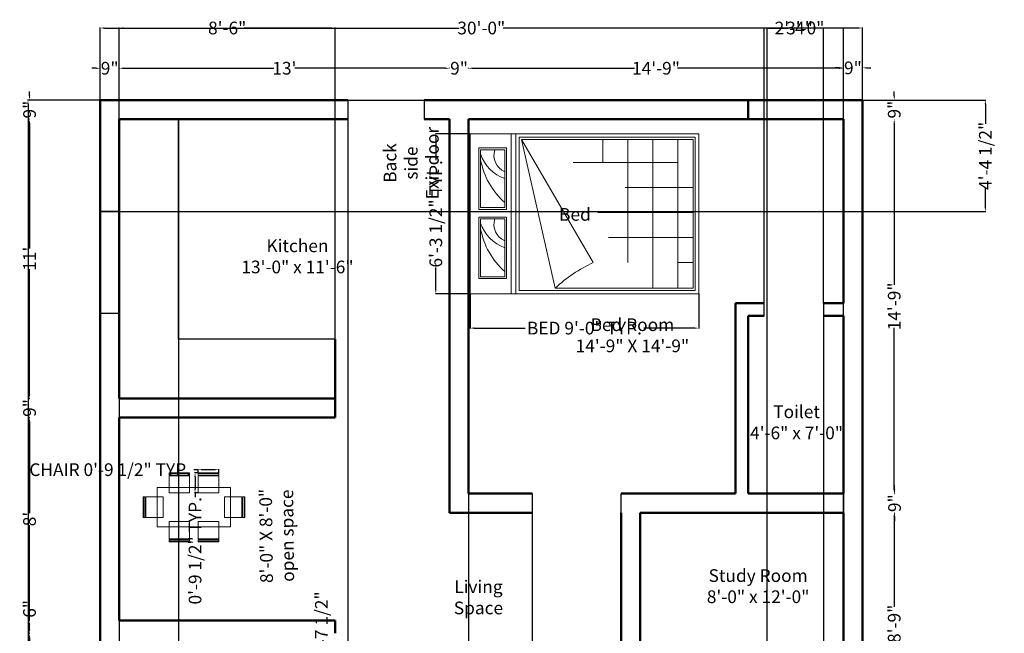
# Model space of a CAD drawing. Units: inches. Extents: x 35 to 505, y 81 to 785.
# Tile 3 of 3: x 40 to 505, y 495 to 785. Entities that reach past the tile are written whole.
import ezdxf

# ---------------------------------------------------------------- set-up
doc = ezdxf.new("R2010")
doc.units = ezdxf.units.IN
doc.header["$MEASUREMENT"] = 0
for name, color, linetype, lineweight in [('A-ANNO-DIMS', 2, 'Continuous', 13), ('A-ANNO-TEXT', 7, 'Continuous', 18), ('A-AREA-IDEN', 7, 'Continuous', 20), ('A-DOOR', 3, 'Continuous', 30), ('A-FLOR-CASE', 8, 'Continuous', 25), ('A-FURN', 6, 'Continuous', 18), ('A-GLAZ', 4, 'Continuous', 25), ('A-WALL', 7, 'Continuous', 50)]:
    doc.layers.add(name, color=color, linetype=linetype, lineweight=lineweight)
doc.styles.get("Standard").update_dxf_attribs({"font": 'arial.ttf'})
doc.dimstyles.get("Standard").update_dxf_attribs({"dimtxt": 6, "dimasz": 2, "dimexe": 0.18, "dimexo": 0.0625, "dimgap": 0.09, "dimtad": 0, "dimdec": 0, "dimzin": 0, "dimdsep": 46, "dimlunit": 4, "dimtxsty": 'Standard', "dimcen": 0.09, "dimadec": 0, "dimazin": 0, "dimtfac": 1, "dimtdec": 0, "dimtofl": 0, "dimtmove": 0, "dimatfit": 3, "dimfxl": 1, "dimtolj": 1, "dimtzin": 0, "dimarcsym": 0})

# ---------------------------------------------------------------- blocks, each defined once
blk = doc.blocks.new('*D6')
at = {"layer": 'A-ANNO-DIMS', "color": 0, "lineweight": -2, "transparency": 16777216}
for p, q in [((44.65, 495.11), (44.53, 495.11)), ((44.71, 493.11), (44.71, 474.08)), ((44.71, 449.11), (44.71, 468.14)), ((44.71, 447.11), (44.89, 447.11))]:
    blk.add_line(p, q, dxfattribs=at)
at = {"layer": 'A-ANNO-DIMS', "color": 0, "transparency": 16777216}
for points in [[(44.38, 493.11), (45.04, 493.11), (44.71, 495.11)], [(44.38, 449.11), (45.04, 449.11), (44.71, 447.11)]]:
    blk.add_solid(points, dxfattribs=at)
at = {"layer": 'Defpoints', "color": 0, "transparency": 16777216}
for p in [(44.71, 495.11), (44.71, 495.11), (44.65, 447.11)]:
    blk.add_point(p, dxfattribs=at)
at = {"layer": 'A-ANNO-DIMS', "color": 0, "transparency": 16777216, "insert": (44.71, 471.11), "char_height": 6, "attachment_point": 5, "rotation": 90}
blk.add_mtext("\\A1;4'", dxfattribs=at)
blk = doc.blocks.new('*D7')
at = {"layer": 'A-ANNO-DIMS', "color": 0, "lineweight": -2, "transparency": 16777216}
for p, q in [((44.71, 501.11), (44.71, 503.11)), ((44.65, 501.11), (44.53, 501.11)), ((44.71, 497.11), (44.71, 499.11)), ((44.77, 495.11), (44.89, 495.11))]:
    blk.add_line(p, q, dxfattribs=at)
at = {"layer": 'A-ANNO-DIMS', "color": 0, "transparency": 16777216}
for points in [[(44.38, 499.11), (45.04, 499.11), (44.71, 501.11)], [(44.38, 497.11), (45.04, 497.11), (44.71, 495.11)]]:
    blk.add_solid(points, dxfattribs=at)
at = {"layer": 'Defpoints', "color": 0, "transparency": 16777216}
for p in [(44.71, 501.11), (44.71, 501.11), (44.71, 495.11)]:
    blk.add_point(p, dxfattribs=at)
at = {"layer": 'A-ANNO-DIMS', "color": 0, "transparency": 16777216, "insert": (44.71, 506.66), "char_height": 6, "attachment_point": 5, "rotation": 90}
blk.add_mtext('\\A1;6"', dxfattribs=at)
blk = doc.blocks.new('*D8')
at = {"layer": 'A-ANNO-DIMS', "color": 0, "lineweight": -2, "transparency": 16777216}
for p, q in [((44.65, 597.11), (44.53, 597.11)), ((44.71, 595.11), (44.71, 551.96)), ((44.71, 503.11), (44.71, 546.25)), ((44.77, 501.11), (44.89, 501.11))]:
    blk.add_line(p, q, dxfattribs=at)
at = {"layer": 'A-ANNO-DIMS', "color": 0, "transparency": 16777216}
for points in [[(44.38, 595.11), (45.04, 595.11), (44.71, 597.11)], [(44.38, 503.11), (45.04, 503.11), (44.71, 501.11)]]:
    blk.add_solid(points, dxfattribs=at)
at = {"layer": 'Defpoints', "color": 0, "transparency": 16777216}
for p in [(44.71, 597.11), (44.71, 597.11), (44.71, 501.11)]:
    blk.add_point(p, dxfattribs=at)
at = {"layer": 'A-ANNO-DIMS', "color": 0, "transparency": 16777216, "insert": (44.71, 549.11), "char_height": 6, "attachment_point": 5, "rotation": 90}
blk.add_mtext("\\A1;8'", dxfattribs=at)
blk = doc.blocks.new('*D9')
at = {"layer": 'A-ANNO-DIMS', "color": 0, "lineweight": -2, "transparency": 16777216}
for p, q in [((44.71, 608.11), (44.71, 610.11)), ((44.65, 606.11), (44.53, 606.11)), ((44.59, 597.11), (44.89, 597.11)), ((44.71, 595.11), (44.71, 593.11))]:
    blk.add_line(p, q, dxfattribs=at)
at = {"layer": 'A-ANNO-DIMS', "color": 0, "transparency": 16777216}
for points in [[(44.38, 608.11), (45.04, 608.11), (44.71, 606.11)], [(44.38, 595.11), (45.04, 595.11), (44.71, 597.11)]]:
    blk.add_solid(points, dxfattribs=at)
at = {"layer": 'Defpoints', "color": 0, "transparency": 16777216}
for p in [(44.71, 606.11), (44.53, 597.11), (44.71, 597.11)]:
    blk.add_point(p, dxfattribs=at)
at = {"layer": 'A-ANNO-DIMS', "color": 0, "transparency": 16777216, "insert": (44.71, 601.61), "char_height": 6, "attachment_point": 5, "rotation": 90}
blk.add_mtext('\\A1;9"', dxfattribs=at)
blk = doc.blocks.new('*D10')
at = {"layer": 'A-ANNO-DIMS', "color": 0, "lineweight": -2, "transparency": 16777216}
for p, q in [((44.65, 738.11), (44.53, 738.11)), ((44.71, 736.11), (44.71, 677.01)), ((44.71, 608.11), (44.71, 667.21)), ((44.77, 606.11), (44.89, 606.11))]:
    blk.add_line(p, q, dxfattribs=at)
at = {"layer": 'A-ANNO-DIMS', "color": 0, "transparency": 16777216}
for points in [[(44.38, 736.11), (45.04, 736.11), (44.71, 738.11)], [(44.38, 608.11), (45.04, 608.11), (44.71, 606.11)]]:
    blk.add_solid(points, dxfattribs=at)
at = {"layer": 'Defpoints', "color": 0, "transparency": 16777216}
for p in [(44.71, 738.11), (44.71, 738.11), (44.71, 606.11)]:
    blk.add_point(p, dxfattribs=at)
at = {"layer": 'A-ANNO-DIMS', "color": 0, "transparency": 16777216, "insert": (44.71, 672.11), "char_height": 6, "attachment_point": 5, "rotation": 90}
blk.add_mtext("\\A1;11'", dxfattribs=at)
blk = doc.blocks.new('*D11')
at = {"layer": 'A-ANNO-DIMS', "color": 0, "lineweight": -2, "transparency": 16777216}
for p, q in [((44.71, 749.11), (44.71, 751.11)), ((44.65, 747.11), (44.53, 747.11)), ((44.65, 738.11), (44.53, 738.11)), ((44.71, 736.11), (44.71, 734.11))]:
    blk.add_line(p, q, dxfattribs=at)
at = {"layer": 'A-ANNO-DIMS', "color": 0, "transparency": 16777216}
for points in [[(44.38, 749.11), (45.04, 749.11), (44.71, 747.11)], [(44.38, 736.11), (45.04, 736.11), (44.71, 738.11)]]:
    blk.add_solid(points, dxfattribs=at)
at = {"layer": 'Defpoints', "color": 0, "transparency": 16777216}
for p in [(44.71, 747.11), (44.71, 738.11), (44.71, 738.11)]:
    blk.add_point(p, dxfattribs=at)
at = {"layer": 'A-ANNO-DIMS', "color": 0, "transparency": 16777216, "insert": (44.71, 742.61), "char_height": 6, "attachment_point": 5, "rotation": 90}
blk.add_mtext('\\A1;9"', dxfattribs=at)
blk = doc.blocks.new('*D12')
at = {"layer": 'A-ANNO-DIMS', "color": 0, "lineweight": -2, "transparency": 16777216}
for p, q in [((76.06, 762.14), (74.06, 762.14)), ((78.06, 747.17), (78.06, 762.32)), ((87.06, 762.21), (87.06, 762.32)), ((89.06, 762.14), (91.06, 762.14))]:
    blk.add_line(p, q, dxfattribs=at)
at = {"layer": 'A-ANNO-DIMS', "color": 0, "transparency": 16777216}
for points in [[(76.06, 762.48), (76.06, 761.81), (78.06, 762.14)], [(89.06, 762.48), (89.06, 761.81), (87.06, 762.14)]]:
    blk.add_solid(points, dxfattribs=at)
at = {"layer": 'Defpoints', "color": 0, "transparency": 16777216}
for p in [(78.06, 762.14), (87.06, 762.14), (78.06, 747.11)]:
    blk.add_point(p, dxfattribs=at)
at = {"layer": 'A-ANNO-DIMS', "color": 0, "transparency": 16777216, "insert": (82.56, 762.14), "char_height": 6, "attachment_point": 5}
blk.add_mtext('\\A1;9"', dxfattribs=at)
blk = doc.blocks.new('*D13')
at = {"layer": 'A-ANNO-DIMS', "color": 0, "lineweight": -2, "transparency": 16777216}
for p, q in [((87.06, 762.26), (87.06, 761.96)), ((89.06, 762.14), (160.16, 762.14)), ((241.06, 762.14), (169.96, 762.14)), ((243.06, 762.21), (243.06, 762.32))]:
    blk.add_line(p, q, dxfattribs=at)
at = {"layer": 'A-ANNO-DIMS', "color": 0, "transparency": 16777216}
for points in [[(89.06, 762.48), (89.06, 761.81), (87.06, 762.14)], [(241.06, 762.48), (241.06, 761.81), (243.06, 762.14)]]:
    blk.add_solid(points, dxfattribs=at)
at = {"layer": 'Defpoints', "color": 0, "transparency": 16777216}
for p in [(87.06, 762.32), (243.06, 762.14), (243.06, 762.14)]:
    blk.add_point(p, dxfattribs=at)
at = {"layer": 'A-ANNO-DIMS', "color": 0, "transparency": 16777216, "insert": (165.06, 762.14), "char_height": 6, "attachment_point": 5}
blk.add_mtext("\\A1;13'", dxfattribs=at)
blk = doc.blocks.new('*D14')
at = {"layer": 'A-ANNO-DIMS', "color": 0, "lineweight": -2, "transparency": 16777216}
for p, q in [((241.06, 762.14), (239.06, 762.14)), ((243.06, 762.21), (243.06, 762.32)), ((252.06, 762.21), (252.06, 762.32)), ((254.06, 762.14), (256.06, 762.14))]:
    blk.add_line(p, q, dxfattribs=at)
at = {"layer": 'A-ANNO-DIMS', "color": 0, "transparency": 16777216}
for points in [[(241.06, 762.48), (241.06, 761.81), (243.06, 762.14)], [(254.06, 762.48), (254.06, 761.81), (252.06, 762.14)]]:
    blk.add_solid(points, dxfattribs=at)
at = {"layer": 'Defpoints', "color": 0, "transparency": 16777216}
for p in [(243.06, 762.14), (252.06, 762.14), (252.06, 762.14)]:
    blk.add_point(p, dxfattribs=at)
at = {"layer": 'A-ANNO-DIMS', "color": 0, "transparency": 16777216, "insert": (247.56, 762.14), "char_height": 6, "attachment_point": 5}
blk.add_mtext('\\A1;9"', dxfattribs=at)
blk = doc.blocks.new('*D15')
at = {"layer": 'A-ANNO-DIMS', "color": 0, "lineweight": -2, "transparency": 16777216}
for p, q in [((252.06, 762.26), (252.06, 761.96)), ((254.06, 762.14), (330.44, 762.14)), ((427.06, 762.14), (350.67, 762.14)), ((429.06, 762.21), (429.06, 762.32))]:
    blk.add_line(p, q, dxfattribs=at)
at = {"layer": 'A-ANNO-DIMS', "color": 0, "transparency": 16777216}
for points in [[(254.06, 762.48), (254.06, 761.81), (252.06, 762.14)], [(427.06, 762.48), (427.06, 761.81), (429.06, 762.14)]]:
    blk.add_solid(points, dxfattribs=at)
at = {"layer": 'Defpoints', "color": 0, "transparency": 16777216}
for p in [(252.06, 762.32), (429.06, 762.14), (429.06, 762.14)]:
    blk.add_point(p, dxfattribs=at)
at = {"layer": 'A-ANNO-DIMS', "color": 0, "transparency": 16777216, "insert": (340.56, 762.14), "char_height": 6, "attachment_point": 5}
blk.add_mtext('\\A1;14\'-9"', dxfattribs=at)
blk = doc.blocks.new('*D16')
at = {"layer": 'A-ANNO-DIMS', "color": 0, "lineweight": -2, "transparency": 16777216}
for p, q in [((427.06, 762.32), (425.06, 762.32)), ((429.06, 762.21), (429.06, 762.5)), ((438.06, 747.17), (438.06, 762.5)), ((440.06, 762.32), (442.06, 762.32))]:
    blk.add_line(p, q, dxfattribs=at)
at = {"layer": 'A-ANNO-DIMS', "color": 0, "transparency": 16777216}
for points in [[(427.06, 762.66), (427.06, 761.99), (429.06, 762.32)], [(440.06, 762.66), (440.06, 761.99), (438.06, 762.32)]]:
    blk.add_solid(points, dxfattribs=at)
at = {"layer": 'Defpoints', "color": 0, "transparency": 16777216}
for p in [(429.06, 762.14), (438.06, 762.32), (438.06, 747.11)]:
    blk.add_point(p, dxfattribs=at)
at = {"layer": 'A-ANNO-DIMS', "color": 0, "transparency": 16777216, "insert": (433.56, 762.32), "char_height": 6, "attachment_point": 5}
blk.add_mtext('\\A1;9"', dxfattribs=at)
blk = doc.blocks.new('*D22')
at = {"layer": 'A-ANNO-DIMS', "color": 0, "lineweight": -2, "transparency": 16777216}
for p, q in [((453.06, 749.11), (453.06, 751.11)), ((438.12, 747.11), (453.24, 747.11)), ((453.06, 736.11), (453.06, 734.11)), ((453.12, 738.11), (453.24, 738.11))]:
    blk.add_line(p, q, dxfattribs=at)
at = {"layer": 'A-ANNO-DIMS', "color": 0, "transparency": 16777216}
for points in [[(452.72, 749.11), (453.39, 749.11), (453.06, 747.11)], [(452.72, 736.11), (453.39, 736.11), (453.06, 738.11)]]:
    blk.add_solid(points, dxfattribs=at)
at = {"layer": 'Defpoints', "color": 0, "transparency": 16777216}
for p in [(438.06, 747.11), (453.06, 738.11), (453.06, 738.11)]:
    blk.add_point(p, dxfattribs=at)
at = {"layer": 'A-ANNO-DIMS', "color": 0, "transparency": 16777216, "insert": (453.06, 742.61), "char_height": 6, "attachment_point": 5, "rotation": 90}
blk.add_mtext('\\A1;9"', dxfattribs=at)
blk = doc.blocks.new('*D23')
at = {"layer": 'A-ANNO-DIMS', "color": 0, "lineweight": -2, "transparency": 16777216}
for p, q in [((453.06, 736.11), (453.06, 659.72)), ((453.12, 738.11), (453.24, 738.11)), ((453.06, 563.11), (453.06, 639.5)), ((453.12, 561.11), (453.24, 561.11))]:
    blk.add_line(p, q, dxfattribs=at)
at = {"layer": 'A-ANNO-DIMS', "color": 0, "transparency": 16777216}
for points in [[(452.72, 736.11), (453.39, 736.11), (453.06, 738.11)], [(452.72, 563.11), (453.39, 563.11), (453.06, 561.11)]]:
    blk.add_solid(points, dxfattribs=at)
at = {"layer": 'Defpoints', "color": 0, "transparency": 16777216}
for p in [(453.06, 738.11), (453.06, 561.11), (453.06, 561.11)]:
    blk.add_point(p, dxfattribs=at)
at = {"layer": 'A-ANNO-DIMS', "color": 0, "transparency": 16777216, "insert": (453.06, 649.61), "char_height": 6, "attachment_point": 5, "rotation": 90}
blk.add_mtext('\\A1;14\'-9"', dxfattribs=at)
blk = doc.blocks.new('*D24')
at = {"layer": 'A-ANNO-DIMS', "color": 0, "lineweight": -2, "transparency": 16777216}
for p, q in [((453.23, 563.11), (453.23, 565.11)), ((453.12, 561.11), (453.41, 561.11)), ((453.12, 552.11), (453.41, 552.11)), ((453.23, 550.11), (453.23, 548.11))]:
    blk.add_line(p, q, dxfattribs=at)
at = {"layer": 'A-ANNO-DIMS', "color": 0, "transparency": 16777216}
for points in [[(452.9, 563.11), (453.56, 563.11), (453.23, 561.11)], [(452.9, 550.11), (453.56, 550.11), (453.23, 552.11)]]:
    blk.add_solid(points, dxfattribs=at)
at = {"layer": 'Defpoints', "color": 0, "transparency": 16777216}
for p in [(453.06, 561.11), (453.06, 552.11), (453.23, 552.11)]:
    blk.add_point(p, dxfattribs=at)
at = {"layer": 'A-ANNO-DIMS', "color": 0, "transparency": 16777216, "insert": (453.23, 556.61), "char_height": 6, "attachment_point": 5, "rotation": 90}
blk.add_mtext('\\A1;9"', dxfattribs=at)
blk = doc.blocks.new('*D25')
at = {"layer": 'A-ANNO-DIMS', "color": 0, "lineweight": -2, "transparency": 16777216}
for p, q in [((453.06, 550.11), (453.06, 507.68)), ((453.12, 552.11), (453.24, 552.11)), ((453.06, 449.11), (453.06, 491.54)), ((453.12, 447.11), (453.24, 447.11))]:
    blk.add_line(p, q, dxfattribs=at)
at = {"layer": 'A-ANNO-DIMS', "color": 0, "transparency": 16777216}
for points in [[(452.72, 550.11), (453.39, 550.11), (453.06, 552.11)], [(452.72, 449.11), (453.39, 449.11), (453.06, 447.11)]]:
    blk.add_solid(points, dxfattribs=at)
at = {"layer": 'Defpoints', "color": 0, "transparency": 16777216}
for p in [(453.06, 552.11), (453.06, 447.11), (453.06, 447.11)]:
    blk.add_point(p, dxfattribs=at)
at = {"layer": 'A-ANNO-DIMS', "color": 0, "transparency": 16777216, "insert": (453.06, 499.61), "char_height": 6, "attachment_point": 5, "rotation": 90}
blk.add_mtext('\\A1;8\'-9"', dxfattribs=at)
blk = doc.blocks.new('bed')
for p, q in [((309.37, 914.01), (309.37, 1021.97)), ((309.37, 1021.97), (384.97, 1021.97)), ((384.97, 1021.97), (384.97, 913.97)), ((316.65, 1017.78), (345.65, 1017.78)), ((316.65, 1004.77), (316.65, 1017.78)), ((317.46, 1016.97), (344.84, 1016.97)), ((317.46, 1005.58), (317.46, 1016.97)), ((344.84, 1016.97), (344.84, 1005.58)), ((345.65, 1017.78), (345.65, 1004.77)), ((349.3, 1017.78), (378.3, 1017.78)), ((349.3, 1004.77), (349.3, 1017.78)), ((350.11, 1016.97), (377.49, 1016.97)), ((350.11, 1005.58), (350.11, 1016.97)), ((377.49, 1016.97), (377.49, 1005.58)), ((378.3, 1017.78), (378.3, 1004.77)), ((345.65, 1004.77), (316.65, 1004.77)), ((344.84, 1005.58), (317.46, 1005.58)), ((378.3, 1004.77), (349.3, 1004.77)), ((377.49, 1005.58), (350.11, 1005.58)), ((309.37, 1002.53), (384.97, 1002.53)), ((309.37, 1000.37), (384.97, 1000.37)), ((310.99, 998.75), (383.35, 998.75)), ((310.99, 915.59), (310.99, 998.75)), ((382.27, 997.67), (312.07, 981.73)), ((382.27, 997.67), (324.17, 963.79)), ((382.27, 997.67), (382.27, 916.67)), ((383.35, 998.75), (383.35, 915.59)), ((312.07, 916.67), (312.07, 981.73)), ((371.46, 923.83), (371.46, 973.35)), ((347.84, 916.67), (347.84, 961.71)), ((371.46, 959.27), (382.27, 959.27)), ((336.02, 916.67), (336.02, 956.58)), ((359.65, 916.67), (359.65, 948.66)), ((324.21, 947.45), (382.27, 947.45)), ((312.07, 935.64), (382.27, 935.64)), ((312.07, 923.83), (382.27, 923.83)), ((324.21, 916.67), (324.21, 923.83)), ((382.27, 916.67), (312.07, 916.67)), ((384.97, 913.97), (309.37, 914.01)), ((383.35, 915.59), (310.99, 915.59))]:
    blk.add_line(p, q)
for centre, radius, start, end in [((346.35, 982.33), 35.21, 100.2734, 138.6774), ((348.52, 999.48), 18.4, 108.0489, 160.6348), ((378.99, 982.33), 35.21, 100.2734, 138.6774), ((381.16, 999.48), 18.4, 108.0489, 160.6348), ((342.22, 1002.22), 8.48, 71.9504, 156.6806), ((374.86, 1002.22), 8.48, 71.9504, 156.6806), ((263.08, 935.62), 67.27, 24.7582, 43.2711)]:
    blk.add_arc(centre, radius, start, end)
blk = doc.blocks.new('CHAIR-DINING')
for p, q in [((0, 9.51, -23.82), (9.73, 9.51, -23.82)), ((0, 1.4, -23.82), (0, 9.51, -23.82)), ((9.73, 9.51, -23.82), (9.73, 1.4, -23.82)), ((9.73, 1.4, -23.82), (0, 1.4, -23.82)), ((9.73, 1.08, -23.82), (0, 1.08, -23.82)), ((0, 1.08, -23.82), (0, 0, -23.82)), ((9.73, 0.33, -23.82), (0, 0.33, -23.82)), ((0, 0, -23.82), (9.73, 0, -23.82)), ((9.73, 0, -23.82), (9.73, 1.08, -23.82))]:
    blk.add_line(p, q)
blk = doc.blocks.new('WIN-48-JAMBS')
for p, q in [((9, 48), (0, 48)), ((0, 0), (9, 0))]:
    blk.add_line(p, q)
blk = doc.blocks.new('DOOR-36-JAMBS')
for p, q in [((0, 9), (0, 0)), ((36, 9), (36, 0))]:
    blk.add_line(p, q)
blk = doc.blocks.new('*D42')
at = {"layer": 'A-ANNO-DIMS', "color": 0, "lineweight": -2, "transparency": 16777216}
for p, q in [((124.34, 572.44), (122.34, 572.44)), ((124.34, 571.04), (124.34, 572.62)), ((132.06, 572.44), (126.34, 572.44)), ((134.06, 571.04), (134.06, 572.62))]:
    blk.add_line(p, q, dxfattribs=at)
at = {"layer": 'A-ANNO-DIMS', "color": 0, "transparency": 16777216}
for points in [[(126.34, 572.77), (126.34, 572.11), (124.34, 572.44)], [(132.06, 572.77), (132.06, 572.11), (134.06, 572.44)]]:
    blk.add_solid(points, dxfattribs=at)
at = {"layer": 'Defpoints', "color": 0, "transparency": 16777216}
for p in [(124.34, 572.44), (124.34, 570.98), (134.06, 570.98)]:
    blk.add_point(p, dxfattribs=at)
at = {"layer": 'A-ANNO-DIMS', "color": 0, "transparency": 16777216, "insert": (82.8, 572.44), "char_height": 6, "attachment_point": 5}
blk.add_mtext('\\A1;CHAIR 0\'-9 1/2" TYP.', dxfattribs=at)
blk = doc.blocks.new('*D43')
at = {"layer": 'A-ANNO-DIMS', "color": 0, "lineweight": -2, "transparency": 16777216}
for p, q in [((124.27, 570.98), (122.7, 570.98)), ((122.88, 568.98), (122.88, 563.48)), ((124.27, 561.48), (122.7, 561.48)), ((122.88, 561.48), (122.88, 559.48))]:
    blk.add_line(p, q, dxfattribs=at)
at = {"layer": 'A-ANNO-DIMS', "color": 0, "transparency": 16777216}
for points in [[(122.54, 568.98), (123.21, 568.98), (122.88, 570.98)], [(122.54, 563.48), (123.21, 563.48), (122.88, 561.48)]]:
    blk.add_solid(points, dxfattribs=at)
at = {"layer": 'Defpoints', "color": 0, "transparency": 16777216}
for p in [(124.34, 570.98), (122.88, 561.48), (124.34, 561.48)]:
    blk.add_point(p, dxfattribs=at)
at = {"layer": 'A-ANNO-DIMS', "color": 0, "transparency": 16777216, "insert": (122.88, 534.11), "char_height": 6, "attachment_point": 5, "rotation": 90}
blk.add_mtext('\\A1;0\'-9 1/2" TYP.', dxfattribs=at)
blk = doc.blocks.new('*D48')
at = {"layer": 'A-ANNO-DIMS', "color": 0, "lineweight": -2, "transparency": 16777216}
for p, q in [((252.77, 655.48), (252.77, 639.16)), ((360.76, 655.48), (360.76, 639.16)), ((254.77, 639.34), (278.74, 639.34)), ((358.76, 639.34), (334.79, 639.34))]:
    blk.add_line(p, q, dxfattribs=at)
at = {"layer": 'A-ANNO-DIMS', "color": 0, "transparency": 16777216}
for points in [[(254.77, 639.67), (254.77, 639.01), (252.77, 639.34)], [(358.76, 639.67), (358.76, 639.01), (360.76, 639.34)]]:
    blk.add_solid(points, dxfattribs=at)
at = {"layer": 'Defpoints', "color": 0, "transparency": 16777216}
for p in [(252.77, 655.54), (360.76, 655.54), (252.77, 639.34)]:
    blk.add_point(p, dxfattribs=at)
at = {"layer": 'A-ANNO-DIMS', "color": 0, "transparency": 16777216, "insert": (306.77, 639.34), "char_height": 6, "attachment_point": 5}
blk.add_mtext('\\A1;BED 9\'-0" TYP.', dxfattribs=at)
blk = doc.blocks.new('*D49')
at = {"layer": 'A-ANNO-DIMS', "color": 0, "lineweight": -2, "transparency": 16777216}
for p, q in [((252.71, 731.14), (236.39, 731.14)), ((236.57, 729.14), (236.57, 718.72)), ((236.57, 657.54), (236.57, 667.95)), ((252.71, 655.54), (236.39, 655.54))]:
    blk.add_line(p, q, dxfattribs=at)
at = {"layer": 'A-ANNO-DIMS', "color": 0, "transparency": 16777216}
for points in [[(236.24, 729.14), (236.9, 729.14), (236.57, 731.14)], [(236.24, 657.54), (236.9, 657.54), (236.57, 655.54)]]:
    blk.add_solid(points, dxfattribs=at)
at = {"layer": 'Defpoints', "color": 0, "transparency": 16777216}
for p in [(236.57, 731.14), (252.77, 731.14), (252.77, 655.54)]:
    blk.add_point(p, dxfattribs=at)
at = {"layer": 'A-ANNO-DIMS', "color": 0, "transparency": 16777216, "insert": (236.57, 693.34), "char_height": 6, "attachment_point": 5, "rotation": 90}
blk.add_mtext('\\A1;6\'-3 1/2" TYP.', dxfattribs=at)
blk = doc.blocks.new('*D50')
at = {"layer": 'A-ANNO-DIMS', "color": 0, "lineweight": -2, "transparency": 16777216}
for p, q in [((182.56, 413.09), (182.56, 415.09)), ((168.89, 413.09), (182.74, 413.09)), ((182.56, 323.55), (182.56, 411.09)), ((168.89, 321.55), (182.74, 321.55))]:
    blk.add_line(p, q, dxfattribs=at)
at = {"layer": 'A-ANNO-DIMS', "color": 0, "transparency": 16777216}
for points in [[(182.23, 411.09), (182.89, 411.09), (182.56, 413.09)], [(182.23, 323.55), (182.89, 323.55), (182.56, 321.55)]]:
    blk.add_solid(points, dxfattribs=at)
at = {"layer": 'Defpoints', "color": 0, "transparency": 16777216}
for p in [(168.83, 413.09), (182.56, 413.09), (168.83, 321.55)]:
    blk.add_point(p, dxfattribs=at)
at = {"layer": 'A-ANNO-DIMS', "color": 0, "transparency": 16777216, "insert": (182.56, 466.23), "char_height": 6, "attachment_point": 5, "rotation": 90}
blk.add_mtext('\\A1;SEATING GROUP 7\'-7 1/2"', dxfattribs=at)
blk = doc.blocks.new('*D52')
at = {"layer": 'A-ANNO-DIMS', "color": 0, "lineweight": -2, "transparency": 16777216}
for p, q in [((78.06, 747.17), (78.06, 781.34)), ((438.06, 747.17), (438.06, 781.34)), ((80.06, 781.16), (247.66, 781.16)), ((436.06, 781.16), (268.45, 781.16))]:
    blk.add_line(p, q, dxfattribs=at)
at = {"layer": 'A-ANNO-DIMS', "color": 0, "transparency": 16777216}
for points in [[(80.06, 781.49), (80.06, 780.83), (78.06, 781.16)], [(436.06, 781.49), (436.06, 780.83), (438.06, 781.16)]]:
    blk.add_solid(points, dxfattribs=at)
at = {"layer": 'Defpoints', "color": 0, "transparency": 16777216}
for p in [(438.06, 781.16), (78.06, 747.11), (438.06, 747.11)]:
    blk.add_point(p, dxfattribs=at)
at = {"layer": 'A-ANNO-DIMS', "color": 0, "transparency": 16777216, "insert": (258.06, 781.16), "char_height": 6, "attachment_point": 5}
blk.add_mtext('\\A1;30\'-0"', dxfattribs=at)
blk = doc.blocks.new('*D53')
at = {"layer": 'A-ANNO-DIMS', "color": 0, "lineweight": -2, "transparency": 16777216}
for p, q in [((77.99, 747.11), (43.83, 747.11)), ((44.01, 745.11), (44.01, 457.5)), ((44.01, 149.11), (44.01, 436.71)), ((77.99, 147.11), (43.83, 147.11))]:
    blk.add_line(p, q, dxfattribs=at)
at = {"layer": 'A-ANNO-DIMS', "color": 0, "transparency": 16777216}
for points in [[(43.67, 745.11), (44.34, 745.11), (44.01, 747.11)], [(43.67, 149.11), (44.34, 149.11), (44.01, 147.11)]]:
    blk.add_solid(points, dxfattribs=at)
at = {"layer": 'Defpoints', "color": 0, "transparency": 16777216}
for p in [(44.01, 747.11), (78.06, 747.11), (78.06, 147.11)]:
    blk.add_point(p, dxfattribs=at)
at = {"layer": 'A-ANNO-DIMS', "color": 0, "transparency": 16777216, "insert": (44.01, 447.11), "char_height": 6, "attachment_point": 5, "rotation": 90}
blk.add_mtext('\\A1;50\'-0"', dxfattribs=at)
blk = doc.blocks.new('*D54')
at = {"layer": 'A-ANNO-DIMS', "color": 0, "lineweight": -2, "transparency": 16777216}
for p, q in [((87.06, 738.05), (87.06, 90.02)), ((195.06, 738.05), (195.06, 90.02)), ((89.06, 90.2), (132.99, 90.2)), ((193.06, 90.2), (149.12, 90.2))]:
    blk.add_line(p, q, dxfattribs=at)
at = {"layer": 'A-ANNO-DIMS', "color": 0, "transparency": 16777216}
for points in [[(89.06, 90.53), (89.06, 89.86), (87.06, 90.2)], [(193.06, 90.53), (193.06, 89.86), (195.06, 90.2)]]:
    blk.add_solid(points, dxfattribs=at)
at = {"layer": 'Defpoints', "color": 0, "transparency": 16777216}
for p in [(87.06, 738.11), (195.06, 738.11), (195.06, 90.2)]:
    blk.add_point(p, dxfattribs=at)
at = {"layer": 'A-ANNO-DIMS', "color": 0, "transparency": 16777216, "insert": (141.06, 90.2), "char_height": 6, "attachment_point": 5}
blk.add_mtext('\\A1;9\'-0"', dxfattribs=at)
blk = doc.blocks.new('*D55')
at = {"layer": 'A-ANNO-DIMS', "color": 0, "lineweight": -2, "transparency": 16777216}
for p, q in [((78.12, 747.11), (496.29, 747.11)), ((496.11, 745.11), (496.11, 735.93)), ((496.11, 696.4), (496.11, 705.58)), ((78.12, 694.4), (496.29, 694.4))]:
    blk.add_line(p, q, dxfattribs=at)
at = {"layer": 'A-ANNO-DIMS', "color": 0, "transparency": 16777216}
for points in [[(495.77, 745.11), (496.44, 745.11), (496.11, 747.11)], [(495.77, 696.4), (496.44, 696.4), (496.11, 694.4)]]:
    blk.add_solid(points, dxfattribs=at)
at = {"layer": 'Defpoints', "color": 0, "transparency": 16777216}
for p in [(78.06, 747.11), (78.06, 694.4), (496.11, 694.4)]:
    blk.add_point(p, dxfattribs=at)
at = {"layer": 'A-ANNO-DIMS', "color": 0, "transparency": 16777216, "insert": (496.11, 720.75), "char_height": 6, "attachment_point": 5, "rotation": 90}
blk.add_mtext('\\A1;4\'-4 1/2"', dxfattribs=at)
blk = doc.blocks.new('*D60')
at = {"layer": 'A-ANNO-DIMS', "color": 0, "lineweight": -2, "transparency": 16777216}
for p, q in [((87.06, 606.17), (87.06, 781.34)), ((189.06, 606.17), (189.06, 781.34)), ((89.06, 781.16), (129.99, 781.16)), ((187.06, 781.16), (146.13, 781.16))]:
    blk.add_line(p, q, dxfattribs=at)
at = {"layer": 'A-ANNO-DIMS', "color": 0, "transparency": 16777216}
for points in [[(89.06, 781.49), (89.06, 780.83), (87.06, 781.16)], [(187.06, 781.49), (187.06, 780.83), (189.06, 781.16)]]:
    blk.add_solid(points, dxfattribs=at)
at = {"layer": 'Defpoints', "color": 0, "transparency": 16777216}
for p in [(189.06, 781.16), (87.06, 606.11), (189.06, 606.11)]:
    blk.add_point(p, dxfattribs=at)
at = {"layer": 'A-ANNO-DIMS', "color": 0, "transparency": 16777216, "insert": (138.06, 781.16), "char_height": 6, "attachment_point": 5}
blk.add_mtext('\\A1;8\'-6"', dxfattribs=at)
blk = doc.blocks.new('*D61')
at = {"layer": 'A-ANNO-DIMS', "color": 0, "lineweight": -2, "transparency": 16777216}
for p, q in [((87.06, 738.05), (87.06, 90.02)), ((115.06, 738.05), (115.06, 90.02)), ((89.06, 90.2), (92.94, 90.2)), ((113.06, 90.2), (109.17, 90.2))]:
    blk.add_line(p, q, dxfattribs=at)
at = {"layer": 'A-ANNO-DIMS', "color": 0, "transparency": 16777216}
for points in [[(89.06, 90.53), (89.06, 89.86), (87.06, 90.2)], [(113.06, 90.53), (113.06, 89.86), (115.06, 90.2)]]:
    blk.add_solid(points, dxfattribs=at)
at = {"layer": 'Defpoints', "color": 0, "transparency": 16777216}
for p in [(87.06, 738.11), (115.06, 738.11), (115.06, 90.2)]:
    blk.add_point(p, dxfattribs=at)
at = {"layer": 'A-ANNO-DIMS', "color": 0, "transparency": 16777216, "insert": (101.06, 90.2), "char_height": 6, "attachment_point": 5}
blk.add_mtext('\\A1;2\'-4"', dxfattribs=at)
blk = doc.blocks.new('*D62')
at = {"layer": 'A-ANNO-DIMS', "color": 0, "lineweight": -2, "transparency": 16777216}
for p, q in [((252.06, 561.05), (252.06, 90.02)), ((282.06, 561.05), (282.06, 90.02)), ((254.06, 90.2), (258.94, 90.2)), ((280.06, 90.2), (275.17, 90.2))]:
    blk.add_line(p, q, dxfattribs=at)
at = {"layer": 'A-ANNO-DIMS', "color": 0, "transparency": 16777216}
for points in [[(254.06, 90.53), (254.06, 89.86), (252.06, 90.2)], [(280.06, 90.53), (280.06, 89.86), (282.06, 90.2)]]:
    blk.add_solid(points, dxfattribs=at)
at = {"layer": 'Defpoints', "color": 0, "transparency": 16777216}
for p in [(252.06, 561.11), (282.06, 561.11), (282.06, 90.2)]:
    blk.add_point(p, dxfattribs=at)
at = {"layer": 'A-ANNO-DIMS', "color": 0, "transparency": 16777216, "insert": (267.06, 90.2), "char_height": 6, "attachment_point": 5}
blk.add_mtext('\\A1;2\'-6"', dxfattribs=at)
blk = doc.blocks.new('*D63')
at = {"layer": 'A-ANNO-DIMS', "color": 0, "lineweight": -2, "transparency": 16777216}
for p, q in [((282.06, 552.05), (282.06, 90.02)), ((324.06, 552.05), (324.06, 90.02)), ((284.06, 90.2), (294.99, 90.2)), ((322.06, 90.2), (311.12, 90.2))]:
    blk.add_line(p, q, dxfattribs=at)
at = {"layer": 'A-ANNO-DIMS', "color": 0, "transparency": 16777216}
for points in [[(284.06, 90.53), (284.06, 89.86), (282.06, 90.2)], [(322.06, 90.53), (322.06, 89.86), (324.06, 90.2)]]:
    blk.add_solid(points, dxfattribs=at)
at = {"layer": 'Defpoints', "color": 0, "transparency": 16777216}
for p in [(282.06, 552.11), (324.06, 552.11), (324.06, 90.2)]:
    blk.add_point(p, dxfattribs=at)
at = {"layer": 'A-ANNO-DIMS', "color": 0, "transparency": 16777216, "insert": (303.06, 90.2), "char_height": 6, "attachment_point": 5}
blk.add_mtext('\\A1;3\'-6"', dxfattribs=at)
blk = doc.blocks.new('*D65')
at = {"layer": 'A-ANNO-DIMS', "color": 0, "lineweight": -2, "transparency": 16777216}
for p, q in [((393.06, 357.17), (393.06, 781.34)), ((429.06, 258.17), (429.06, 781.34)), ((395.06, 781.16), (402.99, 781.16)), ((427.06, 781.16), (419.12, 781.16))]:
    blk.add_line(p, q, dxfattribs=at)
at = {"layer": 'A-ANNO-DIMS', "color": 0, "transparency": 16777216}
for points in [[(395.06, 781.49), (395.06, 780.83), (393.06, 781.16)], [(427.06, 781.49), (427.06, 780.83), (429.06, 781.16)]]:
    blk.add_solid(points, dxfattribs=at)
at = {"layer": 'Defpoints', "color": 0, "transparency": 16777216}
for p in [(429.06, 781.16), (393.06, 357.11), (429.06, 258.11)]:
    blk.add_point(p, dxfattribs=at)
at = {"layer": 'A-ANNO-DIMS', "color": 0, "transparency": 16777216, "insert": (411.06, 781.16), "char_height": 6, "attachment_point": 5}
blk.add_mtext('\\A1;3\'-0"', dxfattribs=at)
blk = doc.blocks.new('*D66')
at = {"layer": 'A-ANNO-DIMS', "color": 0, "lineweight": -2, "transparency": 16777216}
for p, q in [((391.64, 651.17), (391.64, 781.34)), ((419.64, 651.17), (419.64, 781.34)), ((393.64, 781.16), (397.53, 781.16)), ((417.64, 781.16), (413.76, 781.16))]:
    blk.add_line(p, q, dxfattribs=at)
at = {"layer": 'A-ANNO-DIMS', "color": 0, "transparency": 16777216}
for points in [[(393.64, 781.49), (393.64, 780.83), (391.64, 781.16)], [(417.64, 781.49), (417.64, 780.83), (419.64, 781.16)]]:
    blk.add_solid(points, dxfattribs=at)
at = {"layer": 'Defpoints', "color": 0, "transparency": 16777216}
for p in [(419.64, 781.16), (391.64, 651.11), (419.64, 651.11)]:
    blk.add_point(p, dxfattribs=at)
at = {"layer": 'A-ANNO-DIMS', "color": 0, "transparency": 16777216, "insert": (405.64, 781.16), "char_height": 6, "attachment_point": 5}
blk.add_mtext('\\A1;2\'-4"', dxfattribs=at)
blk = doc.blocks.new('*D67')
at = {"layer": 'A-ANNO-DIMS', "color": 0, "lineweight": -2, "transparency": 16777216}
for p, q in [((419.64, 645.05), (419.64, 90.02)), ((429.06, 645.05), (429.06, 90.02)), ((421.64, 90.2), (427.06, 90.2)), ((429.06, 90.2), (431.06, 90.2))]:
    blk.add_line(p, q, dxfattribs=at)
at = {"layer": 'A-ANNO-DIMS', "color": 0, "transparency": 16777216}
for points in [[(421.64, 90.53), (421.64, 89.86), (419.64, 90.2)], [(427.06, 90.53), (427.06, 89.86), (429.06, 90.2)]]:
    blk.add_solid(points, dxfattribs=at)
at = {"layer": 'Defpoints', "color": 0, "transparency": 16777216}
for p in [(419.64, 645.11), (429.06, 645.11), (429.06, 90.2)]:
    blk.add_point(p, dxfattribs=at)
at = {"layer": 'A-ANNO-DIMS', "color": 0, "transparency": 16777216, "insert": (446.11, 90.2), "char_height": 6, "attachment_point": 5}
blk.add_mtext('\\A1;0\'-9 1/2"', dxfattribs=at)

msp = doc.modelspace()

# ---------------------------------------------------------------- linework, layer by layer
at = {"layer": 'A-DOOR'}
for p, q in [((391.64, 645.11), (391.64, 651.11)), ((419.64, 651.11), (419.64, 645.11)), ((282.06, 561.11), (282.06, 552.11)), ((324.06, 552.11), (324.06, 561.11))]:
    msp.add_line(p, q, dxfattribs=at)
at = {"layer": 'A-FLOR-CASE'}
for p, q in [((115.06, 634.11), (115.06, 738.11)), ((189.06, 634.11), (115.06, 634.11))]:
    msp.add_line(p, q, dxfattribs=at)
at = {"layer": 'A-FURN'}
for p, q in [((104.97, 545.43, -23.82), (104.97, 563.96, -23.82)), ((104.97, 563.96, -23.82), (139.7, 563.96, -23.82)), ((139.7, 563.96, -23.82), (139.7, 545.43, -23.82)), ((139.7, 545.43, -23.82), (104.97, 545.43, -23.82))]:
    msp.add_line(p, q, dxfattribs=at)
at = {"layer": 'A-WALL'}
for p, q in [((78.06, 747.11), (195.06, 747.11)), ((78.06, 747.11), (78.06, 147.11)), ((231.06, 747.11), (438.06, 747.11)), ((384.06, 747.11), (384.06, 738.11)), ((438.06, 747.11), (438.06, 249.11)), ((87.06, 738.11), (195.06, 738.11)), ((87.06, 606.11), (87.06, 738.11)), ((231.06, 738.11), (243.06, 738.11)), ((243.06, 738.11), (243.06, 552.11)), ((252.06, 738.11), (252.06, 561.11)), ((252.06, 738.11), (429.06, 738.11)), ((429.06, 738.11), (429.06, 651.11)), ((378.06, 651.11), (378.06, 561.11)), ((378.06, 651.11), (391.64, 651.11)), ((419.64, 651.11), (429.06, 651.11)), ((384.06, 645.11), (391.64, 645.11)), ((384.06, 645.11), (384.06, 561.11)), ((419.64, 645.11), (429.06, 645.11)), ((429.06, 645.11), (429.06, 561.11)), ((189.06, 634.11), (189.06, 597.11)), ((189.06, 606.11), (87.06, 606.11)), ((87.06, 501.11), (87.06, 597.11)), ((189.06, 597.11), (87.06, 597.11)), ((252.06, 561.11), (282.06, 561.11)), ((324.06, 561.11), (378.06, 561.11)), ((384.06, 561.11), (429.06, 561.11)), ((243.06, 552.11), (282.06, 552.11)), ((324.06, 552.11), (324.06, 447.11)), ((333.06, 552.11), (333.06, 447.11)), ((333.06, 552.11), (429.06, 552.11)), ((429.06, 552.11), (429.06, 447.11)), ((189.06, 501.11), (87.06, 501.11)), ((189.06, 501.11), (189.06, 495.11))]:
    msp.add_line(p, q, dxfattribs=at)

# ---------------------------------------------------------------- block references
at = {"layer": 'A-DOOR'}
msp.add_blockref('DOOR-36-JAMBS', (195.06, 738.11), dxfattribs=at)
at = {"layer": 'A-FURN'}
for name, p, rotation in [('bed', (1274.73, 346.17), 90), ('CHAIR-DINING', (120.33, 570.98), 180), ('CHAIR-DINING', (134.06, 570.98), 180), ('CHAIR-DINING', (98.31, 559.58), 270.0000000000061), ('CHAIR-DINING', (146.36, 549.86), 90.0000000000071)]:
    msp.add_blockref(name, p, dxfattribs=dict(at, rotation=rotation))
for p in [(110.6, 538.41), (124.34, 538.41)]:
    msp.add_blockref('CHAIR-DINING', p, dxfattribs=at)
at = {"layer": 'A-GLAZ', "rotation": 180}
msp.add_blockref('WIN-48-JAMBS', (87.06, 694.4), dxfattribs=at)

# ---------------------------------------------------------------- texts
at = {"layer": 'A-ANNO-TEXT', "insert": (211.95, 678.72), "char_height": 6, "attachment_point": 1, "rotation": 90}
msp.add_mtext_dynamic_manual_height_columns('\\pxqc;Back \\Pside\\PExit door', width=77.2296, gutter_width=30, heights=[0], dxfattribs=at)
at = {"layer": 'A-ANNO-TEXT', "insert": (294.79, 696.07), "char_height": 6, "attachment_point": 1}
msp.add_mtext_dynamic_manual_height_columns('Bed', width=25.2815, gutter_width=30, heights=[0], dxfattribs=at)
at = {"layer": 'A-AREA-IDEN', "char_height": 6, "attachment_point": 1}
for s, width, insert in [('\\pxqc;Kitchen\\P13\'-0" x 11\'-6"', 72.7212, (134.89, 681.24)), ('\\pxqc;Bed Room\\P14\'-9" X 14\'-9"', 162.2985, (248.26, 643.95)), ('\\pxqc;Toilet\\P4\'-6" x 7\'-0"', 68.2568, (372.82, 602.82)), ('\\pxqc;Study Room\\P8\'-0" x 12\'-0"', 79.5373, (349.03, 525.39)), ('\\pxqc;Living\\PSpace', 57.1525, (228.14, 520.1))]:
    msp.add_mtext_dynamic_manual_height_columns(s, width=width, gutter_width=30, heights=[0], dxfattribs=dict(at, insert=insert))
at = {"layer": 'A-AREA-IDEN', "insert": (152.88, 589.48), "char_height": 6, "attachment_point": 3, "rotation": 90.658}
msp.add_mtext_dynamic_manual_height_columns('\\pxqc;8\'-0" X 8\'-0"\\Popen space', width=96.7698, gutter_width=30, heights=[0], dxfattribs=at)

# ---------------------------------------------------------------- dimensions: what is measured, and where the dimension line sits
at = {"layer": 'A-ANNO-DIMS'}
for base, p1, p2, override, picture, middle in [((438.06, 781.16), (78.06, 747.11), (438.06, 747.11), {"dimdec": 1, "dimlfac": 1, "dimrnd": 0, "dimzin": 1, "dimdsep": 46, "dimlunit": 4, "dimfrac": 2}, '*D52', (258.06, 781.16)), ((189.06, 781.16), (87.06, 606.11), (189.06, 606.11), {"dimdec": 1, "dimlfac": 1, "dimrnd": 0, "dimzin": 1, "dimdsep": 46, "dimlunit": 4, "dimfrac": 2}, '*D60', (138.06, 781.16)), ((419.64, 781.16), (391.64, 651.11), (419.64, 651.11), {"dimdec": 1, "dimlfac": 1, "dimrnd": 0, "dimzin": 1, "dimdsep": 46, "dimlunit": 4, "dimfrac": 2}, '*D66', (405.64, 781.16)), ((429.06, 781.16), (393.06, 357.11), (429.06, 258.11), {"dimdec": 1, "dimlfac": 1, "dimrnd": 0, "dimzin": 1, "dimdsep": 46, "dimlunit": 4, "dimfrac": 2}, '*D65', (411.06, 781.16)), ((78.06, 762.14), (87.06, 762.14), (78.06, 747.11), {"dimclrd": 0, "dimclre": 0, "dimclrt": 0}, '*D12', (82.56, 762.14)), ((243.06, 762.14), (87.06, 762.32), (243.06, 762.14), {"dimclrd": 0, "dimclre": 0, "dimclrt": 0}, '*D13', (165.06, 762.14)), ((252.06, 762.14), (243.06, 762.14), (252.06, 762.14), {"dimclrd": 0, "dimclre": 0, "dimclrt": 0}, '*D14', (247.56, 762.14)), ((429.06, 762.14), (252.06, 762.32), (429.06, 762.14), {"dimclrd": 0, "dimclre": 0, "dimclrt": 0}, '*D15', (340.56, 762.14)), ((438.06, 762.32), (429.06, 762.14), (438.06, 747.11), {"dimclrd": 0, "dimclre": 0, "dimclrt": 0}, '*D16', (433.56, 762.32)), ((195.06, 90.2), (87.06, 738.11), (195.06, 738.11), {"dimdec": 1, "dimlfac": 1, "dimrnd": 0, "dimzin": 1, "dimdsep": 46, "dimlunit": 4, "dimfrac": 2}, '*D54', (141.06, 90.2)), ((115.06, 90.2), (87.06, 738.11), (115.06, 738.11), {"dimdec": 1, "dimlfac": 1, "dimrnd": 0, "dimzin": 1, "dimdsep": 46, "dimlunit": 4, "dimfrac": 2}, '*D61', (101.06, 90.2)), ((429.06, 90.2), (419.64, 645.11), (429.06, 645.11), {"dimdec": 1, "dimlfac": 1, "dimrnd": 0, "dimzin": 1, "dimdsep": 46, "dimlunit": 4, "dimfrac": 2}, '*D67', (446.11, 90.2)), ((282.06, 90.2), (252.06, 561.11), (282.06, 561.11), {"dimdec": 1, "dimlfac": 1, "dimrnd": 0, "dimzin": 1, "dimdsep": 46, "dimlunit": 4, "dimfrac": 2}, '*D62', (267.06, 90.2)), ((324.06, 90.2), (282.06, 552.11), (324.06, 552.11), {"dimdec": 1, "dimlfac": 1, "dimrnd": 0, "dimzin": 1, "dimdsep": 46, "dimlunit": 4, "dimfrac": 2}, '*D63', (303.06, 90.2))]:
    dim = msp.add_linear_dim(base=base, p1=p1, p2=p2, dimstyle='Standard', override=override, dxfattribs=at)
    dim.commit()
    dim.dimension.update_dxf_attribs({"geometry": picture, "text_midpoint": middle})
for base, p1, p2, override, picture, middle in [((44.71, 738.11), (44.71, 747.11), (44.71, 738.11), {"dimclrd": 0, "dimclre": 0, "dimclrt": 0}, '*D11', (44.71, 742.61)), ((453.06, 738.11), (438.06, 747.11), (453.06, 738.11), {"dimclrd": 0, "dimclre": 0, "dimclrt": 0}, '*D22', (453.06, 742.61)), ((44.01, 747.11), (78.06, 147.11), (78.06, 747.11), {"dimdec": 1, "dimlfac": 1, "dimrnd": 0, "dimzin": 1, "dimdsep": 46, "dimlunit": 4, "dimfrac": 2}, '*D53', (44.01, 447.11)), ((496.11, 694.4), (78.06, 747.11), (78.06, 694.4), {"dimdec": 1, "dimlfac": 1, "dimrnd": 0, "dimzin": 1, "dimdsep": 46, "dimlunit": 4, "dimfrac": 2}, '*D55', (496.11, 720.75)), ((44.71, 738.11), (44.71, 606.11), (44.71, 738.11), {"dimclrd": 0, "dimclre": 0, "dimclrt": 0}, '*D10', (44.71, 672.11)), ((453.06, 561.11), (453.06, 738.11), (453.06, 561.11), {"dimclrd": 0, "dimclre": 0, "dimclrt": 0}, '*D23', (453.06, 649.61)), ((44.71, 597.11), (44.71, 606.11), (44.53, 597.11), {"dimclrd": 0, "dimclre": 0, "dimclrt": 0}, '*D9', (44.71, 601.61)), ((44.71, 597.11), (44.71, 501.11), (44.71, 597.11), {"dimclrd": 0, "dimclre": 0, "dimclrt": 0}, '*D8', (44.71, 549.11)), ((453.23, 552.11), (453.06, 561.11), (453.06, 552.11), {"dimclrd": 0, "dimclre": 0, "dimclrt": 0}, '*D24', (453.23, 556.61)), ((453.06, 447.11), (453.06, 552.11), (453.06, 447.11), {"dimclrd": 0, "dimclre": 0, "dimclrt": 0}, '*D25', (453.06, 499.61)), ((44.71, 501.11), (44.71, 495.11), (44.71, 501.11), {"dimclrd": 0, "dimclre": 0, "dimclrt": 0}, '*D7', (44.71, 506.66)), ((44.71, 495.11), (44.65, 447.11), (44.71, 495.11), {"dimclrd": 0, "dimclre": 0, "dimclrt": 0}, '*D6', (44.71, 471.11))]:
    dim = msp.add_linear_dim(base=base, p1=p1, p2=p2, angle=90, dimstyle='Standard', override=override, dxfattribs=at)
    dim.commit()
    dim.dimension.update_dxf_attribs({"geometry": picture, "text_midpoint": middle})
for base, p1, p2, angle, text, picture, middle in [((236.57, 731.14), (252.77, 655.54), (252.77, 731.14), 90, '<> TYP.', '*D49', (236.57, 693.34)), ((252.77, 639.34), (360.76, 655.54), (252.77, 655.54), 180, 'BED <> TYP.', '*D48', (306.77, 639.34)), ((124.34, 572.44), (134.06, 570.98), (124.34, 570.98), 180, 'CHAIR <> TYP.', '*D42', (82.8, 572.44)), ((122.88, 561.48), (124.34, 570.98), (124.34, 561.48), 270, '<> TYP.', '*D43', (122.88, 534.11)), ((182.56, 413.09), (168.83, 321.55), (168.83, 413.09), 90, 'SEATING GROUP <>', '*D50', (182.56, 466.23))]:
    dim = msp.add_linear_dim(base=base, p1=p1, p2=p2, angle=angle, text=text, dimstyle='Standard', override={"dimdec": 1, "dimlfac": 1, "dimrnd": 0, "dimzin": 1, "dimdsep": 46, "dimlunit": 4, "dimfrac": 2}, dxfattribs=at)
    dim.commit()
    dim.dimension.update_dxf_attribs({"geometry": picture, "text_midpoint": middle})

doc.saveas('drawing.dxf')
